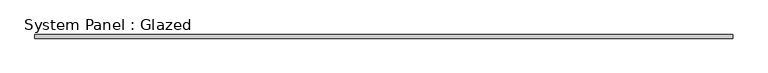
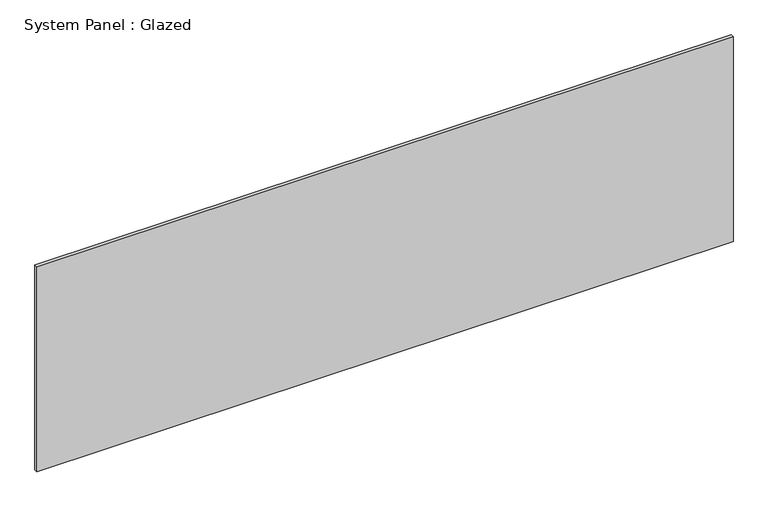
"""IFC4 building model written with IfcOpenShell, lengths in millimetres: plate geometry, System Panel : Glazed."""

from ifc_helpers import new_model, si_unit, origin, origin_with_axes, place, context, project, spatial, polyline, outline, extrude, source, transform, mapped, element, save


def system_panel_glazed_abcfc967(model_context):
    return source(origin(), model_context, "Body", "SweptSolid", [
        extrude(outline(polyline([(2449.1924778, 19.05), (-2449.1924778, 19.05), (-2449.1924778, 44.45), (2449.1924778, 44.45), (2449.1924778, 19.05)])), origin_with_axes(), (0.0, 0.0, 1.0), 1524.0),
    ])


if __name__ == "__main__":
    model = new_model("IFC4")
    model_context = context("Model", 3, world=origin())
    ifc_project = project(units=[si_unit("LENGTHUNIT", "METRE", prefix="MILLI")], contexts=[model_context])
    site = spatial("IfcSite", under=ifc_project)
    building = spatial("IfcBuilding", under=site)
    placement = place(None, origin())
    system_panel_glazed_shape = system_panel_glazed_abcfc967(model_context)
    element("IfcPlate", 1, ObjectType="System Panel : Glazed", at=placement, inside=building, context=model_context, shape_type="MappedRepresentation", body=[
        mapped(system_panel_glazed_shape, transform((0.0, 0.0, 0.0), x_axis=(1.0, 0.0, 0.0), y_axis=(0.0, 1.0, 0.0), z_axis=(0.0, 0.0, 1.0))),
    ])
    save(model, "model.ifc")

# Revit data of these elements
# Type "System Panel : Glazed"
#   Construction Type Id = "GSP4R"
#   Analytic Construction = "1/8 in Pilkington single glazing"
#   Visual Light Transmittance = 0.9
#   Solar Heat Gain Coefficient = 0.86
#   Heat Transfer Coefficient (U) = 1.18115 BTU/(h·ft²·°F)
# Element 1 (IfcPlate, "System Panel : Glazed")
#   Materials on its faces: "Glass"
# Materials
#   "Glass": class "Glass", colour RGB 0 128 192, transparency 0.75, Description = "Soda Lime Glass", Cost = 0
